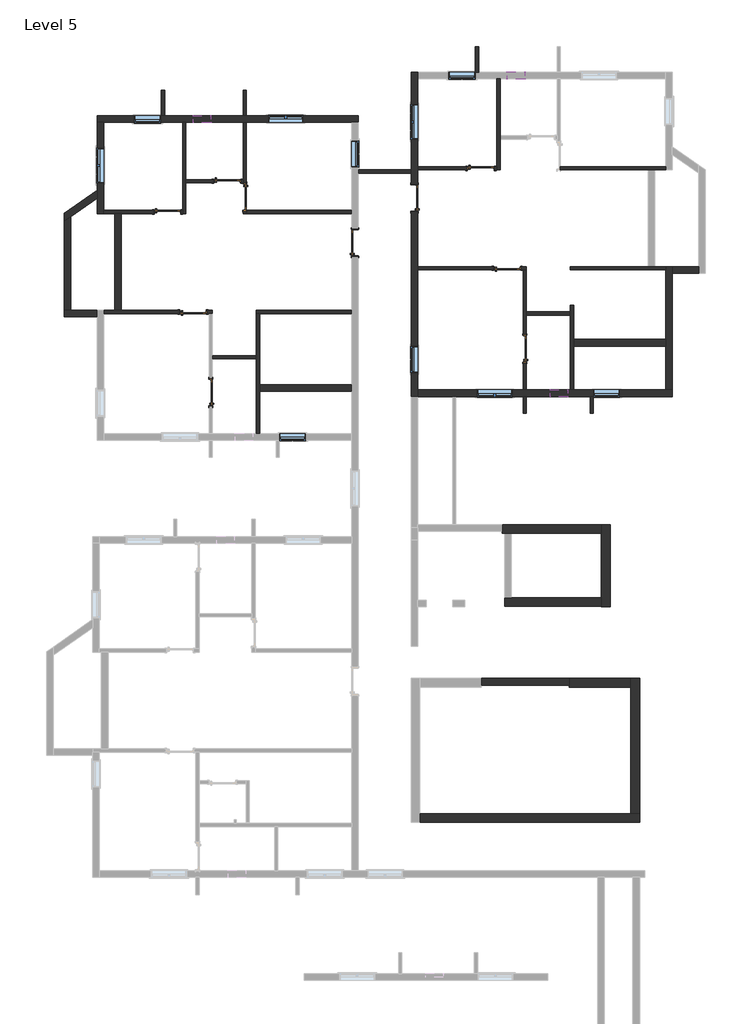
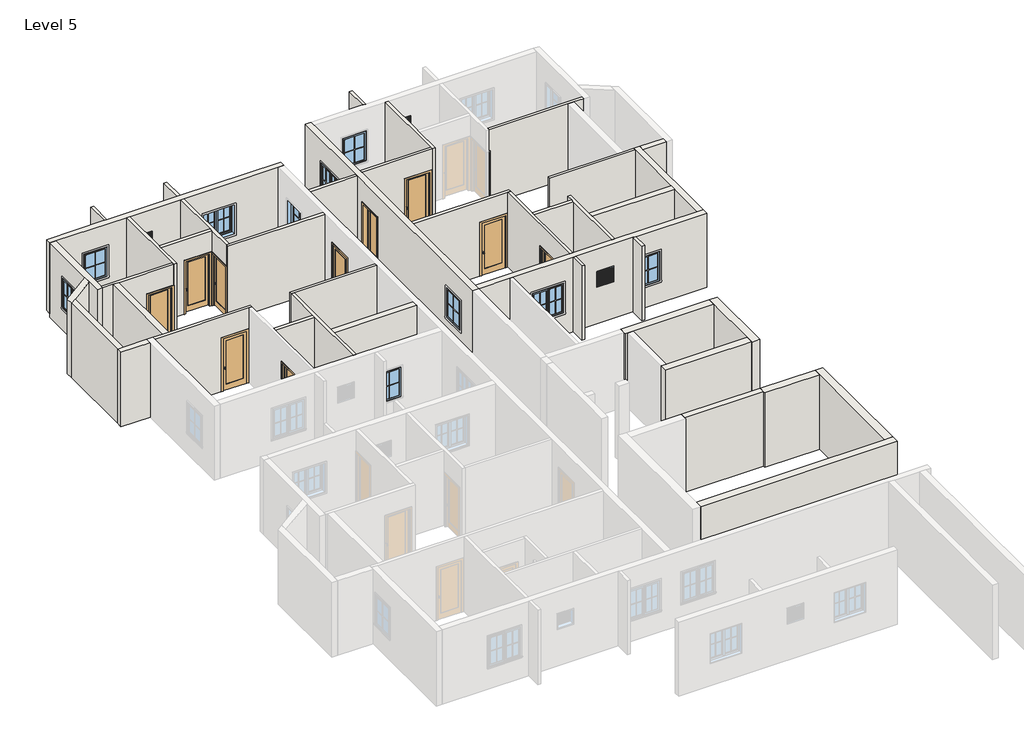
# One storey, part 5 of 7: 42 walls, 13 windows, 10 doors.
"""IFC4 building model written with IfcOpenShell, lengths in millimetres."""

from ifc_helpers import new_model, si_unit, frame, origin, place, context, project, spatial, polyline, outline, extrude, faceted_brep, transform, mapped, element, save
from components import door_3c6ab76a, door_a3feeac7, door_3b97b8e7, door_868ee8a9, window_272f20d6, window_casement_double_4_x_4_af3140d2, window_f2d8fef0

model = new_model("IFC4")

# Units and contexts
model_context = context("Model", 3, world=origin())
ifc_project = project(units=[si_unit("LENGTHUNIT", "METRE", prefix="MILLI")], contexts=[model_context])

# Site, building, storey
site = spatial("IfcSite", under=ifc_project)
building = spatial("IfcBuilding", under=site)
storey = spatial("IfcBuildingStorey", under=building, Name="Level 5", Elevation=6400.8)

# Doors
placement = place(None, origin())
door_shape = door_3c6ab76a(model_context)
element("IfcDoor", 1, ObjectType="Door-Interior-Single-1_Panel-Wood : 2'6\" x 7' door", at=placement, inside=storey, context=model_context, shape_type="MappedRepresentation", body=[
    mapped(door_shape, transform((-10226.9509469, 25492.3711172, 6400.8), x_axis=(1.0, 0.0, 0.0), y_axis=(0.0, 1.0, 0.0), z_axis=(0.0, 0.0, 1.0))),
])
door_2_shape = door_a3feeac7(model_context)
element("IfcDoor", 2, ObjectType="Door-Interior-Single-1_Panel-Wood : 2'6\" x 7' door", at=placement, inside=storey, context=model_context, shape_type="MappedRepresentation", body=[
    mapped(door_2_shape, transform((-10795.2759469, 18161.2961172, 6400.8), x_axis=(0.0, 1.0, 0.0), y_axis=(-1.0, 0.0, 0.0), z_axis=(0.0, 0.0, 1.0))),
])
element("IfcDoor", 3, ObjectType="Door-Interior-Single-1_Panel-Wood : 2'6\" x 7' door", at=placement, inside=storey, context=model_context, shape_type="MappedRepresentation", body=[
    mapped(door_2_shape, transform((101.3240531, 19674.7755084, 6400.8), x_axis=(0.0, 1.0, 0.0), y_axis=(-1.0, 0.0, 0.0), z_axis=(0.0, 0.0, 1.0))),
])
element("IfcDoor", 4, ObjectType="Door-Interior-Single-1_Panel-Wood : 36\" x 84\"", at=placement, inside=storey, context=model_context, shape_type="MappedRepresentation", body=[
    mapped(door_shape, transform((-12297.0509469, 24425.5711172, 6400.8), x_axis=(1.0, 0.0, 0.0), y_axis=(0.0, 1.0, 0.0), z_axis=(0.0, 0.0, 1.0))),
])
element("IfcDoor", 5, ObjectType="Door-Interior-Single-1_Panel-Wood : 36\" x 84\"", at=placement, inside=storey, context=model_context, shape_type="MappedRepresentation", body=[
    mapped(door_shape, transform((-9614.1759469, 24936.7461172, 6400.8), x_axis=(0.0, -1.0, 0.0), y_axis=(1.0, 0.0, 0.0), z_axis=(0.0, 0.0, 1.0))),
])
element("IfcDoor", 6, ObjectType="Door-Interior-Single-1_Panel-Wood : 36\" x 84\"", at=placement, inside=storey, context=model_context, shape_type="MappedRepresentation", body=[
    mapped(door_shape, transform((-1425.8509469, 25939.0505084, 6400.8), x_axis=(1.0, 0.0, 0.0), y_axis=(0.0, 1.0, 0.0), z_axis=(0.0, 0.0, 1.0))),
])
door_3_shape = door_3b97b8e7(model_context)
element("IfcDoor", 7, ObjectType="Door-Interior-Single-1_Panel-Wood : 36\" x 84\"", at=placement, inside=storey, context=model_context, shape_type="MappedRepresentation", body=[
    mapped(door_3_shape, transform((-5791.4759469, 23355.5961172, 6400.8), x_axis=(0.0, 1.0, 0.0), y_axis=(-1.0, 0.0, 0.0), z_axis=(0.0, 0.0, 1.0))),
])
element("IfcDoor", 8, ObjectType="Door-Interior-Single-1_Panel-Wood : 36\" x 84\"", at=placement, inside=storey, context=model_context, shape_type="MappedRepresentation", body=[
    mapped(door_2_shape, transform((-11408.0509469, 20952.1211172, 6400.8), x_axis=(1.0, 0.0, 0.0), y_axis=(0.0, 1.0, 0.0), z_axis=(0.0, 0.0, 1.0))),
])
element("IfcDoor", 9, ObjectType="Door-Interior-Single-1_Panel-Wood : 36\" x 84\"", at=placement, inside=storey, context=model_context, shape_type="MappedRepresentation", body=[
    mapped(door_2_shape, transform((-511.4509469, 22465.6005084, 6400.8), x_axis=(1.0, 0.0, 0.0), y_axis=(0.0, 1.0, 0.0), z_axis=(0.0, 0.0, 1.0))),
])
door_4_shape = door_868ee8a9(model_context)
element("IfcDoor", 10, ObjectType="Door-Interior-Single-1_Panel-Wood : 36\" x 84\"", at=placement, inside=storey, context=model_context, shape_type="MappedRepresentation", body=[
    mapped(door_4_shape, transform((-3727.7259469, 24907.1755084, 6400.8), x_axis=(0.0, 1.0, 0.0), y_axis=(-1.0, 0.0, 0.0), z_axis=(0.0, 0.0, 1.0))),
])

# Walls
element("IfcWall", 11, ObjectType="1' feet", at=placement, inside=storey, context=model_context, shape_type="Brep", body=[
    faceted_brep([(-682.9009469, 13266.6182723, 6400.8), (2758.7990531, 13266.6182723, 6400.8), (2758.7990531, 13266.6182723, 9448.8), (-682.9009469, 13266.6182723, 9448.8), (-682.9009469, 13571.4182723, 6400.8), (-682.9009469, 13571.4182723, 9448.8), (2758.7990531, 13571.4182723, 9448.8), (2758.7990531, 13571.4182723, 6400.8), (-682.9009469, 13342.8182723, 6400.8), (-682.9009469, 13342.8182723, 9448.8)], [[[0, 1, 2, 3]], [[4, 5, 6, 7]], [[1, 0, 8, 4, 7]], [[3, 2, 6, 5, 9]], [[0, 3, 9, 5, 4, 8]], [[2, 1, 7, 6]]]),
])
element("IfcWall", 12, ObjectType="1' feet", at=placement, inside=storey, context=model_context, shape_type="Brep", body=[
    faceted_brep([(3063.5990531, 10726.6182723, 6400.8), (3063.5990531, 13571.4182723, 6400.8), (3063.5990531, 13571.4182723, 9448.8), (3063.5990531, 10726.6182723, 9448.8), (2758.7990531, 10726.6182723, 6400.8), (2758.7990531, 10726.6182723, 9448.8), (2758.7990531, 10739.3182723, 9448.8), (2758.7990531, 11044.1182723, 9448.8), (2758.7990531, 13266.6182723, 9448.8), (2758.7990531, 13571.4182723, 9448.8), (2758.7990531, 13571.4182723, 6400.8), (2758.7990531, 13266.6182723, 6400.8), (2758.7990531, 11044.1182723, 6400.8), (2758.7990531, 10739.3182723, 6400.8)], [[[0, 1, 2, 3]], [[4, 5, 6, 7, 8, 9, 10, 11, 12, 13]], [[1, 0, 4, 13, 12, 11, 10]], [[3, 2, 9, 8, 7, 6, 5]], [[0, 3, 5, 4]], [[2, 1, 10, 9]]]),
])
element("IfcWall", 13, ObjectType="1' feet", at=placement, inside=storey, context=model_context, shape_type="Brep", body=[
    faceted_brep([(2758.7990531, 11044.1182723, 6400.8), (-365.4009469, 11044.1182723, 6400.8), (-594.0009469, 11044.1182723, 6400.8), (-594.0009469, 11044.1182723, 9448.8), (-365.4009469, 11044.1182723, 9448.8), (2758.7990531, 11044.1182723, 9448.8), (2758.7990531, 10739.3182723, 6400.8), (2758.7990531, 10739.3182723, 9448.8), (-594.0009469, 10739.3182723, 9448.8), (-594.0009469, 10739.3182723, 6400.8)], [[[0, 1, 2, 3, 4, 5]], [[6, 7, 8, 9]], [[2, 1, 0, 6, 9]], [[5, 4, 3, 8, 7]], [[0, 5, 7, 6]], [[3, 2, 9, 8]]]),
])
element("IfcWall", 14, ObjectType="1' feet", at=placement, inside=storey, context=model_context, shape_type="Brep", body=[
    faceted_brep([(-3540.4009469, 3245.1461172, 6400.8), (4079.5990531, 3245.1461172, 6400.8), (4079.5990531, 3245.1461172, 9448.8), (-3540.4009469, 3245.1461172, 9448.8), (-3540.4009469, 3549.9461172, 6400.8), (-3540.4009469, 3549.9461172, 9448.8), (3774.7990531, 3549.9461172, 9448.8), (4079.5990531, 3549.9461172, 9448.8), (4079.5990531, 3549.9461172, 6400.8), (3774.7990531, 3549.9461172, 6400.8)], [[[0, 1, 2, 3]], [[4, 5, 6, 7, 8, 9]], [[1, 0, 4, 9, 8]], [[3, 2, 7, 6, 5]], [[2, 1, 8, 7]], [[0, 3, 5, 4]]]),
])
element("IfcWall", 15, ObjectType="1' feet", at=placement, inside=storey, context=model_context, shape_type="Brep", body=[
    faceted_brep([(4079.5990531, 3549.9461172, 6400.8), (4079.5990531, 8236.2461172, 6400.8), (4079.5990531, 8236.2461172, 9448.8), (4079.5990531, 3549.9461172, 9448.8), (3774.7990531, 3549.9461172, 6400.8), (3774.7990531, 3549.9461172, 9448.8), (3774.7990531, 7931.4461172, 9448.8), (3774.7990531, 8236.2461172, 9448.8), (3774.7990531, 8236.2461172, 6400.8), (3774.7990531, 7931.4461172, 6400.8)], [[[0, 1, 2, 3]], [[4, 5, 6, 7, 8, 9]], [[1, 0, 4, 9, 8]], [[3, 2, 7, 6, 5]], [[0, 3, 5, 4]], [[2, 1, 8, 7]]]),
])
element("IfcWall", 16, ObjectType="1' feet", at=placement, inside=storey, context=model_context, shape_type="Brep", body=[
    faceted_brep([(1641.1990531, 7931.4461172, 6400.8), (3774.7990531, 7931.4461172, 6400.8), (3774.7990531, 7931.4461172, 9448.8), (1641.1990531, 7931.4461172, 9448.8), (1641.1990531, 8236.2461172, 6400.8), (1641.1990531, 8236.2461172, 9448.8), (3774.7990531, 8236.2461172, 9448.8), (3774.7990531, 8236.2461172, 6400.8), (1641.1990531, 8007.6461172, 6400.8), (1641.1990531, 8007.6461172, 9448.8)], [[[0, 1, 2, 3]], [[4, 5, 6, 7]], [[1, 0, 8, 4, 7]], [[3, 2, 6, 5, 9]], [[0, 3, 9, 5, 4, 8]], [[2, 1, 7, 6]]]),
])
element("IfcWall", 17, ObjectType="4.5\" wall", at=placement, inside=storey, context=model_context, shape_type="Brep", body=[
    faceted_brep([(-11655.7009469, 24365.2461172, 6400.8), (-11655.7009469, 25432.0461172, 6400.8), (-11655.7009469, 25546.3461172, 6400.8), (-11655.7009469, 27527.5461172, 6400.8), (-11655.7009469, 27527.5461172, 9448.8), (-11655.7009469, 25546.3461172, 9448.8), (-11655.7009469, 25432.0461172, 9448.8), (-11655.7009469, 24365.2461172, 9448.8), (-11770.0009469, 24365.2461172, 6400.8), (-11770.0009469, 24365.2461172, 9448.8), (-11770.0009469, 24479.5461172, 9448.8), (-11770.0009469, 27527.5461172, 9448.8), (-11770.0009469, 27527.5461172, 6400.8), (-11770.0009469, 24479.5461172, 6400.8)], [[[0, 1, 2, 3, 4, 5, 6, 7]], [[8, 9, 10, 11, 12, 13]], [[3, 2, 1, 0, 8, 13, 12]], [[7, 6, 5, 4, 11, 10, 9]], [[4, 3, 12, 11]], [[0, 7, 9, 8]]]),
])
element("IfcWall", 18, ObjectType="4.5\" wall", at=placement, inside=storey, context=model_context, shape_type="SweptSolid", body=[
    extrude(outline(polyline([(9448.8, -9674.5009469), (9448.8, -11655.7009469), (6400.8, -11655.7009469), (6400.8, -10709.5509469), (8559.8, -10709.5509469), (8559.8, -9744.3509469), (6400.8, -9744.3509469), (6400.8, -9674.5009469), (9448.8, -9674.5009469)])), frame((0.0, 25432.0461172, 0.0), z_axis=(0.0, 1.0, 0.0), x_axis=(0.0, 0.0, 1.0)), (0.0, 0.0, 1.0), 114.3),
])
element("IfcWall", 19, ObjectType="4.5\" wall", at=placement, inside=storey, context=model_context, shape_type="Brep", body=[
    faceted_brep([(-11770.0009469, 24365.2461172, 9448.8), (-13903.6009469, 24365.2461172, 9448.8), (-14132.2009469, 24365.2461172, 9448.8), (-14513.2009469, 24365.2461172, 9448.8), (-14513.2009469, 24365.2461172, 6400.8), (-14132.2009469, 24365.2461172, 6400.8), (-13903.6009469, 24365.2461172, 6400.8), (-12779.6509469, 24365.2461172, 6400.8), (-12779.6509469, 24365.2461172, 8559.8), (-11814.4509469, 24365.2461172, 8559.8), (-11814.4509469, 24365.2461172, 6400.8), (-11770.0009469, 24365.2461172, 6400.8), (-14513.2009469, 24479.5461172, 9448.8), (-11770.0009469, 24479.5461172, 9448.8), (-11770.0009469, 24479.5461172, 6400.8), (-11814.4509469, 24479.5461172, 6400.8), (-11814.4509469, 24479.5461172, 8559.8), (-12779.6509469, 24479.5461172, 8559.8), (-12779.6509469, 24479.5461172, 6400.8), (-14513.2009469, 24479.5461172, 6400.8)], [[[0, 1, 2, 3, 4, 5, 6, 7, 8, 9, 10, 11]], [[12, 13, 14, 15, 16, 17, 18, 19]], [[4, 19, 18, 7, 6, 5]], [[14, 11, 10, 15]], [[3, 2, 1, 0, 13, 12]], [[4, 3, 12, 19]], [[0, 11, 14, 13]], [[9, 16, 15, 10]], [[16, 9, 8, 17]], [[17, 8, 7, 18]]]),
])
element("IfcWall", 20, ObjectType="4.5\" wall", at=placement, inside=storey, context=model_context, shape_type="Brep", body=[
    faceted_brep([(-9674.5009469, 24479.5461172, 9448.8), (-9560.2009469, 24479.5461172, 9448.8), (-5902.6009469, 24479.5461172, 9448.8), (-5902.6009469, 24479.5461172, 6400.8), (-9560.2009469, 24479.5461172, 6400.8), (-9560.2009469, 24479.5461172, 8559.8), (-9674.5009469, 24479.5461172, 8559.8), (-9674.5009469, 24365.2461172, 6400.8), (-5902.6009469, 24365.2461172, 6400.8), (-5902.6009469, 24365.2461172, 9448.8), (-9674.5009469, 24365.2461172, 9448.8), (-9674.5009469, 24454.1461172, 6400.8), (-9560.2009469, 24454.1461172, 6400.8), (-9674.5009469, 24454.1461172, 8559.8), (-9560.2009469, 24454.1461172, 8559.8)], [[[0, 1, 2, 3, 4, 5, 6]], [[7, 8, 9, 10]], [[8, 7, 11, 12, 4, 3]], [[2, 1, 0, 10, 9]], [[7, 10, 0, 6, 13, 11]], [[3, 2, 9, 8]], [[12, 14, 5, 4]], [[14, 12, 11, 13]], [[14, 13, 6, 5]]]),
])
element("IfcWall", 21, ObjectType="4.5\" wall", at=placement, inside=storey, context=model_context, shape_type="Brep", body=[
    faceted_brep([(-5902.6009469, 21012.4461172, 6400.8), (-9217.3009469, 21012.4461172, 6400.8), (-9217.3009469, 21012.4461172, 9448.8), (-5902.6009469, 21012.4461172, 9448.8), (-5902.6009469, 20898.1461172, 6400.8), (-5902.6009469, 20898.1461172, 9448.8), (-9103.0009469, 20898.1461172, 9448.8), (-9217.3009469, 20898.1461172, 9448.8), (-9217.3009469, 20898.1461172, 6400.8), (-9103.0009469, 20898.1461172, 6400.8)], [[[0, 1, 2, 3]], [[4, 5, 6, 7, 8, 9]], [[1, 0, 4, 9, 8]], [[3, 2, 7, 6, 5]], [[0, 3, 5, 4]], [[2, 1, 8, 7]]]),
])
element("IfcWall", 22, ObjectType="4.5\" wall", at=placement, inside=storey, context=model_context, shape_type="Brep", body=[
    faceted_brep([(-14513.2009469, 21012.4461172, 9448.8), (-14132.2009469, 21012.4461172, 9448.8), (-13903.6009469, 21012.4461172, 9448.8), (-10741.3009469, 21012.4461172, 9448.8), (-10741.3009469, 21012.4461172, 6400.8), (-10925.4509469, 21012.4461172, 6400.8), (-10925.4509469, 21012.4461172, 8559.8), (-11890.6509469, 21012.4461172, 8559.8), (-11890.6509469, 21012.4461172, 6400.8), (-13903.6009469, 21012.4461172, 6400.8), (-14132.2009469, 21012.4461172, 6400.8), (-14513.2009469, 21012.4461172, 6400.8), (-10741.3009469, 20898.1461172, 9448.8), (-10855.6009469, 20898.1461172, 9448.8), (-14513.2009469, 20898.1461172, 9448.8), (-14513.2009469, 20898.1461172, 6400.8), (-11890.6509469, 20898.1461172, 6400.8), (-11890.6509469, 20898.1461172, 8559.8), (-10925.4509469, 20898.1461172, 8559.8), (-10925.4509469, 20898.1461172, 6400.8), (-10855.6009469, 20898.1461172, 6400.8), (-10741.3009469, 20898.1461172, 6400.8)], [[[0, 1, 2, 3, 4, 5, 6, 7, 8, 9, 10, 11]], [[12, 13, 14, 15, 16, 17, 18, 19, 20, 21]], [[15, 11, 10, 9, 8, 16]], [[4, 21, 20, 19, 5]], [[3, 2, 1, 0, 14, 13, 12]], [[0, 11, 15, 14]], [[4, 3, 12, 21]], [[18, 6, 5, 19]], [[6, 18, 17, 7]], [[7, 17, 16, 8]]]),
])
element("IfcWall", 23, ObjectType="4.5\" wall", at=placement, inside=storey, context=model_context, shape_type="Brep", body=[
    faceted_brep([(-9560.2009469, 27527.5461172, 9448.8), (-9560.2009469, 24479.5461172, 9448.8), (-9560.2009469, 24479.5461172, 8559.8), (-9560.2009469, 25419.3461172, 8559.8), (-9560.2009469, 25419.3461172, 6400.8), (-9560.2009469, 27527.5461172, 6400.8), (-9674.5009469, 24479.5461172, 9448.8), (-9674.5009469, 25432.0461172, 9448.8), (-9674.5009469, 25546.3461172, 9448.8), (-9674.5009469, 27527.5461172, 9448.8), (-9674.5009469, 27527.5461172, 6400.8), (-9674.5009469, 25546.3461172, 6400.8), (-9674.5009469, 25432.0461172, 6400.8), (-9674.5009469, 25419.3461172, 6400.8), (-9674.5009469, 25419.3461172, 8559.8), (-9674.5009469, 24479.5461172, 8559.8)], [[[0, 1, 2, 3, 4, 5]], [[6, 7, 8, 9, 10, 11, 12, 13, 14, 15]], [[10, 5, 4, 13, 12, 11]], [[1, 0, 9, 8, 7, 6]], [[0, 5, 10, 9]], [[1, 6, 15, 2]], [[14, 3, 2, 15]], [[3, 14, 13, 4]]]),
])
element("IfcWall", 24, ObjectType="4.5\" wall", at=placement, inside=storey, context=model_context, shape_type="SweptSolid", body=[
    extrude(outline(polyline([(-9217.3009469, 19323.3461172), (-10741.3009469, 19323.3461172), (-10741.3009469, 19437.6461172), (-9217.3009469, 19437.6461172), (-9217.3009469, 19323.3461172)])), frame((0.0, 0.0, 6400.8), z_axis=(0.0, 0.0, 1.0), x_axis=(1.0, 0.0, 0.0)), (0.0, 0.0, 1.0), 3048.0),
])
element("IfcWall", 25, ObjectType="4.5\" wall", at=placement, inside=storey, context=model_context, shape_type="Brep", body=[
    faceted_brep([(-9217.3009469, 20898.1461172, 6400.8), (-9217.3009469, 19437.6461172, 6400.8), (-9217.3009469, 19323.3461172, 6400.8), (-9217.3009469, 16732.5461172, 6400.8), (-9217.3009469, 16732.5461172, 9448.8), (-9217.3009469, 19323.3461172, 9448.8), (-9217.3009469, 19437.6461172, 9448.8), (-9217.3009469, 20898.1461172, 9448.8), (-9103.0009469, 20898.1461172, 6400.8), (-9103.0009469, 20898.1461172, 9448.8), (-9103.0009469, 18434.3461172, 9448.8), (-9103.0009469, 18205.7461172, 9448.8), (-9103.0009469, 16732.5461172, 9448.8), (-9103.0009469, 16732.5461172, 6400.8), (-9103.0009469, 18205.7461172, 6400.8), (-9103.0009469, 18434.3461172, 6400.8)], [[[0, 1, 2, 3, 4, 5, 6, 7]], [[8, 9, 10, 11, 12, 13, 14, 15]], [[3, 2, 1, 0, 8, 15, 14, 13]], [[7, 6, 5, 4, 12, 11, 10, 9]], [[0, 7, 9, 8]], [[4, 3, 13, 12]]]),
])
element("IfcWall", 26, ObjectType="4.5\" wall", at=placement, inside=storey, context=model_context, shape_type="SweptSolid", body=[
    extrude(outline(polyline([(-5674.0009469, 25878.7255084), (-3845.2009469, 25878.7255084), (-3845.2009469, 25764.4255084), (-5674.0009469, 25764.4255084), (-5674.0009469, 25878.7255084)])), frame((0.0, 0.0, 6400.8), z_axis=(0.0, 0.0, 1.0), x_axis=(1.0, 0.0, 0.0)), (0.0, 0.0, 1.0), 3048.0),
])
element("IfcWall", 27, ObjectType="4.5\" wall", at=placement, inside=storey, context=model_context, shape_type="Brep", body=[
    faceted_brep([(-759.1009469, 25878.7255084, 6400.8), (-759.1009469, 26945.5255084, 6400.8), (-759.1009469, 27059.8255084, 6400.8), (-759.1009469, 29041.0255084, 6400.8), (-759.1009469, 29041.0255084, 9448.8), (-759.1009469, 27059.8255084, 9448.8), (-759.1009469, 26945.5255084, 9448.8), (-759.1009469, 25878.7255084, 9448.8), (-873.4009469, 25878.7255084, 6400.8), (-873.4009469, 25878.7255084, 9448.8), (-873.4009469, 25993.0255084, 9448.8), (-873.4009469, 29041.0255084, 9448.8), (-873.4009469, 29041.0255084, 6400.8), (-873.4009469, 25993.0255084, 6400.8)], [[[0, 1, 2, 3, 4, 5, 6, 7]], [[8, 9, 10, 11, 12, 13]], [[3, 2, 1, 0, 8, 13, 12]], [[7, 6, 5, 4, 11, 10, 9]], [[4, 3, 12, 11]], [[0, 7, 9, 8]]]),
])
element("IfcWall", 28, ObjectType="4.5\" wall", at=placement, inside=storey, context=model_context, shape_type="SweptSolid", body=[
    extrude(outline(polyline([(9448.8, -873.4009469), (9448.8, -3616.6009469), (6400.8, -3616.6009469), (6400.8, -1908.4509469), (8559.8, -1908.4509469), (8559.8, -943.2509469), (6400.8, -943.2509469), (6400.8, -873.4009469), (9448.8, -873.4009469)])), frame((0.0, 25878.7255084, 0.0), z_axis=(0.0, 1.0, 0.0), x_axis=(0.0, 0.0, 1.0)), (0.0, 0.0, 1.0), 114.3),
])
element("IfcWall", 29, ObjectType="4.5\" wall", at=placement, inside=storey, context=model_context, shape_type="Brep", body=[
    faceted_brep([(4993.9990531, 25993.0255084, 6400.8), (1336.3990531, 25993.0255084, 6400.8), (1336.3990531, 25993.0255084, 9448.8), (4993.9990531, 25993.0255084, 9448.8), (4993.9990531, 25878.7255084, 6400.8), (4993.9990531, 25878.7255084, 9448.8), (4612.9990531, 25878.7255084, 9448.8), (4384.3990531, 25878.7255084, 9448.8), (1336.3990531, 25878.7255084, 9448.8), (1336.3990531, 25878.7255084, 6400.8), (4384.3990531, 25878.7255084, 6400.8), (4612.9990531, 25878.7255084, 6400.8)], [[[0, 1, 2, 3]], [[4, 5, 6, 7, 8, 9, 10, 11]], [[1, 0, 4, 11, 10, 9]], [[3, 2, 8, 7, 6, 5]], [[2, 1, 9, 8]], [[0, 3, 5, 4]]]),
])
element("IfcWall", 30, ObjectType="4.5\" wall", at=placement, inside=storey, context=model_context, shape_type="Brep", body=[
    faceted_brep([(4993.9990531, 22525.9255084, 6400.8), (4612.9990531, 22525.9255084, 6400.8), (4384.3990531, 22525.9255084, 6400.8), (1679.2990531, 22525.9255084, 6400.8), (1679.2990531, 22525.9255084, 9448.8), (4384.3990531, 22525.9255084, 9448.8), (4612.9990531, 22525.9255084, 9448.8), (4993.9990531, 22525.9255084, 9448.8), (4993.9990531, 22411.6255084, 6400.8), (4993.9990531, 22411.6255084, 9448.8), (1679.2990531, 22411.6255084, 9448.8), (1679.2990531, 22411.6255084, 6400.8)], [[[0, 1, 2, 3, 4, 5, 6, 7]], [[8, 9, 10, 11]], [[3, 2, 1, 0, 8, 11]], [[4, 3, 11, 10]], [[7, 6, 5, 4, 10, 9]], [[0, 7, 9, 8]]]),
])
element("IfcWall", 31, ObjectType="4.5\" wall", at=placement, inside=storey, context=model_context, shape_type="Brep", body=[
    faceted_brep([(155.2990531, 22411.6255084, 9448.8), (40.9990531, 22411.6255084, 9448.8), (-3616.6009469, 22411.6255084, 9448.8), (-3616.6009469, 22411.6255084, 6400.8), (-994.0509469, 22411.6255084, 6400.8), (-994.0509469, 22411.6255084, 8559.8), (-28.8509469, 22411.6255084, 8559.8), (-28.8509469, 22411.6255084, 6400.8), (40.9990531, 22411.6255084, 6400.8), (155.2990531, 22411.6255084, 6400.8), (-3616.6009469, 22525.9255084, 9448.8), (155.2990531, 22525.9255084, 9448.8), (155.2990531, 22525.9255084, 6400.8), (-28.8509469, 22525.9255084, 6400.8), (-28.8509469, 22525.9255084, 8559.8), (-994.0509469, 22525.9255084, 8559.8), (-994.0509469, 22525.9255084, 6400.8), (-3616.6009469, 22525.9255084, 6400.8)], [[[0, 1, 2, 3, 4, 5, 6, 7, 8, 9]], [[10, 11, 12, 13, 14, 15, 16, 17]], [[3, 17, 16, 4]], [[12, 9, 8, 7, 13]], [[2, 1, 0, 11, 10]], [[3, 2, 10, 17]], [[0, 9, 12, 11]], [[6, 14, 13, 7]], [[14, 6, 5, 15]], [[15, 5, 4, 16]]]),
])
element("IfcWall", 32, ObjectType="4.5\" wall", at=placement, inside=storey, context=model_context, shape_type="Brep", body=[
    faceted_brep([(155.2990531, 22411.6255084, 9448.8), (155.2990531, 20951.1255084, 9448.8), (155.2990531, 20836.8255084, 9448.8), (155.2990531, 18246.0255084, 9448.8), (155.2990531, 18246.0255084, 6400.8), (155.2990531, 19192.1755084, 6400.8), (155.2990531, 19192.1755084, 8559.8), (155.2990531, 20157.3755084, 8559.8), (155.2990531, 20157.3755084, 6400.8), (155.2990531, 20836.8255084, 6400.8), (155.2990531, 20951.1255084, 6400.8), (155.2990531, 22411.6255084, 6400.8), (40.9990531, 18246.0255084, 9448.8), (40.9990531, 22411.6255084, 9448.8), (40.9990531, 22411.6255084, 6400.8), (40.9990531, 20157.3755084, 6400.8), (40.9990531, 20157.3755084, 8559.8), (40.9990531, 19192.1755084, 8559.8), (40.9990531, 19192.1755084, 6400.8), (40.9990531, 18246.0255084, 6400.8)], [[[0, 1, 2, 3, 4, 5, 6, 7, 8, 9, 10, 11]], [[12, 13, 14, 15, 16, 17, 18, 19]], [[14, 11, 10, 9, 8, 15]], [[4, 19, 18, 5]], [[3, 2, 1, 0, 13, 12]], [[0, 11, 14, 13]], [[4, 3, 12, 19]], [[7, 16, 15, 8]], [[16, 7, 6, 17]], [[17, 6, 5, 18]]]),
])
element("IfcWall", 33, ObjectType="4.5\" wall", at=placement, inside=storey, context=model_context, shape_type="Brep", body=[
    faceted_brep([(1679.2990531, 21192.4255084, 6400.8), (1679.2990531, 20951.1255084, 6400.8), (1679.2990531, 20836.8255084, 6400.8), (1679.2990531, 18246.0255084, 6400.8), (1679.2990531, 18246.0255084, 9448.8), (1679.2990531, 20836.8255084, 9448.8), (1679.2990531, 20951.1255084, 9448.8), (1679.2990531, 21192.4255084, 9448.8), (1793.5990531, 21192.4255084, 6400.8), (1793.5990531, 21192.4255084, 9448.8), (1793.5990531, 19998.6255084, 9448.8), (1793.5990531, 19770.0255084, 9448.8), (1793.5990531, 18246.0255084, 9448.8), (1793.5990531, 18246.0255084, 6400.8), (1793.5990531, 19770.0255084, 6400.8), (1793.5990531, 19998.6255084, 6400.8)], [[[0, 1, 2, 3, 4, 5, 6, 7]], [[8, 9, 10, 11, 12, 13, 14, 15]], [[3, 2, 1, 0, 8, 15, 14, 13]], [[7, 6, 5, 4, 12, 11, 10, 9]], [[0, 7, 9, 8]], [[4, 3, 13, 12]]]),
])
element("IfcWall", 34, ObjectType="4.5\" wall", at=placement, inside=storey, context=model_context, shape_type="SweptSolid", body=[
    extrude(outline(polyline([(155.2990531, 20951.1255084), (1679.2990531, 20951.1255084), (1679.2990531, 20836.8255084), (155.2990531, 20836.8255084), (155.2990531, 20951.1255084)])), frame((0.0, 0.0, 6400.8), z_axis=(0.0, 0.0, 1.0), x_axis=(1.0, 0.0, 0.0)), (0.0, 0.0, 1.0), 3048.0),
])
element("IfcWall", 35, ObjectType="4.5\" wall", at=placement, inside=storey, context=model_context, shape_type="Brep", body=[
    faceted_brep([(-1617.8862554, 30161.6889788, 6400.8), (-1617.8862554, 29269.6255084, 6400.8), (-1617.8862554, 29269.6255084, 7315.2), (-1617.8862554, 29269.6255084, 8534.4), (-1617.8862554, 29269.6255084, 9448.8), (-1617.8862554, 30161.6889788, 9448.8), (-1503.5862554, 30161.6889788, 6400.8), (-1503.5862554, 30161.6889788, 9448.8), (-1503.5862554, 29269.6255084, 9448.8), (-1503.5862554, 29269.6255084, 6400.8)], [[[0, 1, 2, 3, 4, 5]], [[6, 7, 8, 9]], [[1, 0, 6, 9]], [[5, 4, 8, 7]], [[0, 5, 7, 6]], [[4, 3, 2, 1, 9, 8]]]),
])
element("IfcWall", 36, ObjectType="4.5\" wall", at=placement, inside=storey, context=model_context, shape_type="SweptSolid", body=[
    extrude(outline(polyline([(40.9990531, 17431.8689406), (40.9990531, 18017.4255084), (155.2990531, 18017.4255084), (155.2990531, 17431.8689406), (40.9990531, 17431.8689406)])), frame((0.0, 0.0, 6400.8), z_axis=(0.0, 0.0, 1.0), x_axis=(1.0, 0.0, 0.0)), (0.0, 0.0, 1.0), 3048.0),
])
element("IfcWall", 37, ObjectType="4.5\" wall", at=placement, inside=storey, context=model_context, shape_type="Brep", body=[
    faceted_brep([(2365.0990531, 18017.4255084, 6400.8), (2365.0990531, 17431.8689406, 6400.8), (2365.0990531, 17431.8689406, 9448.8), (2365.0990531, 18017.4255084, 9448.8), (2479.3990531, 18017.4255084, 6400.8), (2479.3990531, 18017.4255084, 7315.2), (2479.3990531, 18017.4255084, 8534.4), (2479.3990531, 18017.4255084, 9448.8), (2479.3990531, 17431.8689406, 9448.8), (2479.3990531, 17431.8689406, 6400.8)], [[[0, 1, 2, 3]], [[4, 5, 6, 7, 8, 9]], [[1, 0, 4, 9]], [[2, 1, 9, 8]], [[3, 2, 8, 7]], [[0, 3, 7, 6, 5, 4]]]),
])
element("IfcWall", 38, ObjectType="4.5\" wall", at=placement, inside=storey, context=model_context, shape_type="SweptSolid", body=[
    extrude(outline(polyline([(-12514.4862554, 27756.1461172), (-12514.4862554, 28648.2095876), (-12400.1862554, 28648.2095876), (-12400.1862554, 27756.1461172), (-12514.4862554, 27756.1461172)])), frame((0.0, 0.0, 6400.8), z_axis=(0.0, 0.0, 1.0), x_axis=(1.0, 0.0, 0.0)), (0.0, 0.0, 1.0), 3048.0),
])
element("IfcWall", 39, ObjectType="4.5\" wall", at=placement, inside=storey, context=model_context, shape_type="SweptSolid", body=[
    extrude(outline(polyline([(-9560.2009469, 28648.2095876), (-9560.2009469, 27756.1461172), (-9674.5009469, 27756.1461172), (-9674.5009469, 28648.2095876), (-9560.2009469, 28648.2095876)])), frame((0.0, 0.0, 6400.8), z_axis=(0.0, 0.0, 1.0), x_axis=(1.0, 0.0, 0.0)), (0.0, 0.0, 1.0), 3048.0),
])
element("IfcWall", 40, ObjectType="9\"", at=placement, inside=storey, context=model_context, shape_type="Brep", body=[
    faceted_brep([(-5674.0009469, 27756.1461172, 6553.2), (-14741.8009469, 27756.1461172, 6553.2), (-14741.8009469, 27756.1461172, 9448.8), (-12514.4862554, 27756.1461172, 9448.8), (-12400.1862554, 27756.1461172, 9448.8), (-9674.5009469, 27756.1461172, 9448.8), (-9560.2009469, 27756.1461172, 9448.8), (-5674.0009469, 27756.1461172, 9448.8), (-10798.4509469, 27756.1461172, 8534.4), (-11408.0509469, 27756.1461172, 8534.4), (-11408.0509469, 27756.1461172, 7924.8), (-10798.4509469, 27756.1461172, 7924.8), (-13447.9362554, 27756.1461172, 8534.4), (-13447.9362554, 27756.1461172, 7315.2), (-12533.5362554, 27756.1461172, 7315.2), (-12533.5362554, 27756.1461172, 8534.4), (-7585.3509469, 27756.1461172, 8534.4), (-8804.5509469, 27756.1461172, 8534.4), (-8804.5509469, 27756.1461172, 7315.2), (-7585.3509469, 27756.1461172, 7315.2), (-5674.0009469, 27527.5461172, 6553.2), (-5674.0009469, 27527.5461172, 9448.8), (-5902.6009469, 27527.5461172, 9448.8), (-9560.2009469, 27527.5461172, 9448.8), (-9674.5009469, 27527.5461172, 9448.8), (-11655.7009469, 27527.5461172, 9448.8), (-11770.0009469, 27527.5461172, 9448.8), (-14513.2009469, 27527.5461172, 9448.8), (-14741.8009469, 27527.5461172, 9448.8), (-14741.8009469, 27527.5461172, 6553.2), (-10798.4509469, 27527.5461172, 8534.4), (-10798.4509469, 27527.5461172, 7924.8), (-11408.0509469, 27527.5461172, 7924.8), (-11408.0509469, 27527.5461172, 8534.4), (-13447.9362554, 27527.5461172, 8534.4), (-12533.5362554, 27527.5461172, 8534.4), (-12533.5362554, 27527.5461172, 7315.2), (-13447.9362554, 27527.5461172, 7315.2), (-7585.3509469, 27527.5461172, 8534.4), (-7585.3509469, 27527.5461172, 7315.2), (-8804.5509469, 27527.5461172, 7315.2), (-8804.5509469, 27527.5461172, 8534.4)], [[[0, 1, 2, 3, 4, 5, 6, 7], [8, 9, 10, 11], [12, 13, 14, 15], [16, 17, 18, 19]], [[20, 21, 22, 23, 24, 25, 26, 27, 28, 29], [30, 31, 32, 33], [34, 35, 36, 37], [38, 39, 40, 41]], [[1, 0, 20, 29]], [[7, 6, 5, 4, 3, 2, 28, 27, 26, 25, 24, 23, 22, 21]], [[2, 1, 29, 28]], [[0, 7, 21, 20]], [[31, 30, 8, 11]], [[32, 31, 11, 10]], [[33, 32, 10, 9]], [[30, 33, 9, 8]], [[13, 12, 34, 37]], [[14, 13, 37, 36]], [[15, 14, 36, 35]], [[12, 15, 35, 34]], [[39, 38, 16, 19]], [[40, 39, 19, 18]], [[41, 40, 18, 17]], [[38, 41, 17, 16]]]),
])
element("IfcWall", 41, ObjectType="9\"", at=placement, inside=storey, context=model_context, shape_type="Brep", body=[
    faceted_brep([(-14741.8009469, 27527.5461172, 6400.8), (-14741.8009469, 25177.6879786, 6400.8), (-14741.8009469, 24898.6461172, 6400.8), (-14741.8009469, 24365.2461172, 6400.8), (-14741.8009469, 24365.2461172, 9448.8), (-14741.8009469, 24898.6461172, 9448.8), (-14741.8009469, 25177.6879786, 9448.8), (-14741.8009469, 27527.5461172, 9448.8), (-14741.8009469, 27527.5461172, 6553.2), (-14741.8009469, 26641.7211172, 8534.4), (-14741.8009469, 25422.5211172, 8534.4), (-14741.8009469, 25422.5211172, 7315.2), (-14741.8009469, 26641.7211172, 7315.2), (-14513.2009469, 27527.5461172, 6400.8), (-14513.2009469, 27527.5461172, 9448.8), (-14513.2009469, 24479.5461172, 9448.8), (-14513.2009469, 24365.2461172, 9448.8), (-14513.2009469, 24365.2461172, 6400.8), (-14513.2009469, 24479.5461172, 6400.8), (-14513.2009469, 26641.7211172, 8534.4), (-14513.2009469, 26641.7211172, 7315.2), (-14513.2009469, 25422.5211172, 7315.2), (-14513.2009469, 25422.5211172, 8534.4)], [[[0, 1, 2, 3, 4, 5, 6, 7, 8], [9, 10, 11, 12]], [[13, 14, 15, 16, 17, 18], [19, 20, 21, 22]], [[3, 2, 1, 0, 13, 18, 17]], [[7, 6, 5, 4, 16, 15, 14]], [[0, 8, 7, 14, 13]], [[4, 3, 17, 16]], [[20, 19, 9, 12]], [[21, 20, 12, 11]], [[22, 21, 11, 10]], [[19, 22, 10, 9]]]),
])
element("IfcWall", 42, ObjectType="9\"", at=placement, inside=storey, context=model_context, shape_type="SweptSolid", body=[
    extrude(outline(polyline([(-13903.6009469, 24365.2461172), (-13903.6009469, 21012.4461172), (-14132.2009469, 21012.4461172), (-14132.2009469, 24365.2461172), (-13903.6009469, 24365.2461172)])), frame((0.0, 0.0, 6400.8), z_axis=(0.0, 0.0, 1.0), x_axis=(1.0, 0.0, 0.0)), (0.0, 0.0, 1.0), 3048.0),
])
element("IfcWall", 43, ObjectType="9\"", at=placement, inside=storey, context=model_context, shape_type="SweptSolid", body=[
    extrude(outline(polyline([(-5902.6009469, 18205.7461172), (-9103.0009469, 18205.7461172), (-9103.0009469, 18434.3461172), (-5902.6009469, 18434.3461172), (-5902.6009469, 18205.7461172)])), frame((0.0, 0.0, 6400.8), z_axis=(0.0, 0.0, 1.0), x_axis=(1.0, 0.0, 0.0)), (0.0, 0.0, 1.0), 3048.0),
])
element("IfcWall", 44, ObjectType="9\"", at=placement, inside=storey, context=model_context, shape_type="Brep", body=[
    faceted_brep([(-3616.6009469, 29269.6255084, 9448.8), (-3616.6009469, 29041.0255084, 9448.8), (-3616.6009469, 25993.0255084, 9448.8), (-3616.6009469, 25878.7255084, 9448.8), (-3616.6009469, 22525.9255084, 9448.8), (-3616.6009469, 22411.6255084, 9448.8), (-3616.6009469, 18246.0255084, 9448.8), (-3616.6009469, 18017.4255084, 9448.8), (-3616.6009469, 18017.4255084, 6400.8), (-3616.6009469, 18246.0255084, 6400.8), (-3616.6009469, 22411.6255084, 6400.8), (-3616.6009469, 22525.9255084, 6400.8), (-3616.6009469, 24424.5755084, 6400.8), (-3616.6009469, 24424.5755084, 8559.8), (-3616.6009469, 25389.7755084, 8559.8), (-3616.6009469, 25389.7755084, 6400.8), (-3616.6009469, 25878.7255084, 6400.8), (-3616.6009469, 25993.0255084, 6400.8), (-3616.6009469, 29041.0255084, 6400.8), (-3616.6009469, 29269.6255084, 6400.8), (-3616.6009469, 19757.3255084, 8534.4), (-3616.6009469, 19757.3255084, 7315.2), (-3616.6009469, 18842.9255084, 7315.2), (-3616.6009469, 18842.9255084, 8534.4), (-3616.6009469, 28155.2005084, 8534.4), (-3616.6009469, 28155.2005084, 7315.2), (-3616.6009469, 26936.0005084, 7315.2), (-3616.6009469, 26936.0005084, 8534.4), (-3845.2009469, 18017.4255084, 9448.8), (-3845.2009469, 25764.4255084, 9448.8), (-3845.2009469, 25878.7255084, 9448.8), (-3845.2009469, 29269.6255084, 9448.8), (-3845.2009469, 29269.6255084, 6400.8), (-3845.2009469, 25878.7255084, 6400.8), (-3845.2009469, 25764.4255084, 6400.8), (-3845.2009469, 25389.7755084, 6400.8), (-3845.2009469, 25389.7755084, 8559.8), (-3845.2009469, 24424.5755084, 8559.8), (-3845.2009469, 24424.5755084, 6400.8), (-3845.2009469, 18017.4255084, 6400.8), (-3845.2009469, 19757.3255084, 8534.4), (-3845.2009469, 18842.9255084, 8534.4), (-3845.2009469, 18842.9255084, 7315.2), (-3845.2009469, 19757.3255084, 7315.2), (-3845.2009469, 28155.2005084, 8534.4), (-3845.2009469, 26936.0005084, 8534.4), (-3845.2009469, 26936.0005084, 7315.2), (-3845.2009469, 28155.2005084, 7315.2)], [[[0, 1, 2, 3, 4, 5, 6, 7, 8, 9, 10, 11, 12, 13, 14, 15, 16, 17, 18, 19], [20, 21, 22, 23], [24, 25, 26, 27]], [[28, 29, 30, 31, 32, 33, 34, 35, 36, 37, 38, 39], [40, 41, 42, 43], [44, 45, 46, 47]], [[32, 19, 18, 17, 16, 15, 35, 34, 33]], [[8, 39, 38, 12, 11, 10, 9]], [[7, 6, 5, 4, 3, 2, 1, 0, 31, 30, 29, 28]], [[0, 19, 32, 31]], [[8, 7, 28, 39]], [[14, 36, 35, 15]], [[36, 14, 13, 37]], [[37, 13, 12, 38]], [[21, 20, 40, 43]], [[22, 21, 43, 42]], [[23, 22, 42, 41]], [[20, 23, 41, 40]], [[25, 24, 44, 47]], [[26, 25, 47, 46]], [[27, 26, 46, 45]], [[24, 27, 45, 44]]]),
])
element("IfcWall", 45, ObjectType="9\"", at=placement, inside=storey, context=model_context, shape_type="Brep", body=[
    faceted_brep([(-3616.6009469, 18017.4255084, 6400.8), (-2402.381873, 18017.4255084, 6400.8), (-2288.081873, 18017.4255084, 6400.8), (40.9990531, 18017.4255084, 6400.8), (155.2990531, 18017.4255084, 6400.8), (2365.0990531, 18017.4255084, 6400.8), (2479.3990531, 18017.4255084, 6400.8), (5222.5990531, 18017.4255084, 6400.8), (5222.5990531, 18017.4255084, 9448.8), (2479.3990531, 18017.4255084, 9448.8), (2365.0990531, 18017.4255084, 9448.8), (155.2990531, 18017.4255084, 9448.8), (40.9990531, 18017.4255084, 9448.8), (-2288.081873, 18017.4255084, 9448.8), (-2402.381873, 18017.4255084, 9448.8), (-3616.6009469, 18017.4255084, 9448.8), (1590.3990531, 18017.4255084, 8534.4), (1590.3990531, 18017.4255084, 7924.8), (980.7990531, 18017.4255084, 7924.8), (980.7990531, 18017.4255084, 8534.4), (2479.3990531, 18017.4255084, 8534.4), (3393.7990531, 18017.4255084, 8534.4), (3393.7990531, 18017.4255084, 7315.2), (2479.3990531, 18017.4255084, 7315.2), (-1552.8509469, 18017.4255084, 8534.4), (-333.6509469, 18017.4255084, 8534.4), (-333.6509469, 18017.4255084, 7315.2), (-1552.8509469, 18017.4255084, 7315.2), (-3616.6009469, 18246.0255084, 6400.8), (-3616.6009469, 18246.0255084, 9448.8), (40.9990531, 18246.0255084, 9448.8), (155.2990531, 18246.0255084, 9448.8), (1679.2990531, 18246.0255084, 9448.8), (1793.5990531, 18246.0255084, 9448.8), (4993.9990531, 18246.0255084, 9448.8), (5222.5990531, 18246.0255084, 9448.8), (5222.5990531, 18246.0255084, 6400.8), (4993.9990531, 18246.0255084, 6400.8), (1793.5990531, 18246.0255084, 6400.8), (1679.2990531, 18246.0255084, 6400.8), (155.2990531, 18246.0255084, 6400.8), (40.9990531, 18246.0255084, 6400.8), (1590.3990531, 18246.0255084, 8534.4), (980.7990531, 18246.0255084, 8534.4), (980.7990531, 18246.0255084, 7924.8), (1590.3990531, 18246.0255084, 7924.8), (2479.3990531, 18246.0255084, 8534.4), (2479.3990531, 18246.0255084, 7315.2), (3393.7990531, 18246.0255084, 7315.2), (3393.7990531, 18246.0255084, 8534.4), (-1552.8509469, 18246.0255084, 8534.4), (-1552.8509469, 18246.0255084, 7315.2), (-333.6509469, 18246.0255084, 7315.2), (-333.6509469, 18246.0255084, 8534.4)], [[[0, 1, 2, 3, 4, 5, 6, 7, 8, 9, 10, 11, 12, 13, 14, 15], [16, 17, 18, 19], [20, 21, 22, 23], [24, 25, 26, 27]], [[28, 29, 30, 31, 32, 33, 34, 35, 36, 37, 38, 39, 40, 41], [42, 43, 44, 45], [46, 47, 48, 49], [50, 51, 52, 53]], [[7, 6, 5, 4, 3, 2, 1, 0, 28, 41, 40, 39, 38, 37, 36]], [[15, 14, 13, 12, 11, 10, 9, 8, 35, 34, 33, 32, 31, 30, 29]], [[0, 15, 29, 28]], [[8, 7, 36, 35]], [[17, 16, 42, 45]], [[18, 17, 45, 44]], [[19, 18, 44, 43]], [[16, 19, 43, 42]], [[47, 46, 20, 23]], [[48, 47, 23, 22]], [[49, 48, 22, 21]], [[46, 49, 21, 20]], [[51, 50, 24, 27]], [[52, 51, 27, 26]], [[53, 52, 26, 25]], [[50, 53, 25, 24]]]),
])
element("IfcWall", 46, ObjectType="9\"", at=placement, inside=storey, context=model_context, shape_type="Brep", body=[
    faceted_brep([(4993.9990531, 22525.9255084, 6400.8), (4993.9990531, 22411.6255084, 6400.8), (4993.9990531, 19998.6255084, 6400.8), (4993.9990531, 19770.0255084, 6400.8), (4993.9990531, 18246.0255084, 6400.8), (4993.9990531, 18246.0255084, 9448.8), (4993.9990531, 19770.0255084, 9448.8), (4993.9990531, 19998.6255084, 9448.8), (4993.9990531, 22411.6255084, 9448.8), (4993.9990531, 22525.9255084, 9448.8), (5222.5990531, 22525.9255084, 6400.8), (5222.5990531, 22525.9255084, 9448.8), (5222.5990531, 22297.3255084, 9448.8), (5222.5990531, 18246.0255084, 9448.8), (5222.5990531, 18246.0255084, 6400.8), (5222.5990531, 22297.3255084, 6400.8)], [[[0, 1, 2, 3, 4, 5, 6, 7, 8, 9]], [[10, 11, 12, 13, 14, 15]], [[4, 3, 2, 1, 0, 10, 15, 14]], [[9, 8, 7, 6, 5, 13, 12, 11]], [[5, 4, 14, 13]], [[0, 9, 11, 10]]]),
])
element("IfcWall", 47, ObjectType="9\"", at=placement, inside=storey, context=model_context, shape_type="SweptSolid", body=[
    extrude(outline(polyline([(4993.9990531, 19770.0255084), (1793.5990531, 19770.0255084), (1793.5990531, 19998.6255084), (4993.9990531, 19998.6255084), (4993.9990531, 19770.0255084)])), frame((0.0, 0.0, 6400.8), z_axis=(0.0, 0.0, 1.0), x_axis=(1.0, 0.0, 0.0)), (0.0, 0.0, 1.0), 3048.0),
])
element("IfcWall", 48, ObjectType="9\"", at=placement, inside=storey, context=model_context, shape_type="SweptSolid", body=[
    extrude(outline(polyline([(1641.1990531, 8007.6461172), (-1406.8009469, 8007.6461172), (-1406.8009469, 8236.2461172), (1641.1990531, 8236.2461172), (1641.1990531, 8007.6461172)])), frame((0.0, 0.0, 6400.8), z_axis=(0.0, 0.0, 1.0), x_axis=(1.0, 0.0, 0.0)), (0.0, 0.0, 1.0), 3048.0),
])
element("IfcWall", 49, ObjectType="9\"", at=placement, inside=storey, context=model_context, shape_type="Brep", body=[
    faceted_brep([(-14741.8009469, 21012.4461172, 6400.8), (-15656.2009469, 21012.4461172, 6400.8), (-15884.8009469, 21012.4461172, 6400.8), (-15884.8009469, 21012.4461172, 9448.8), (-15656.2009469, 21012.4461172, 9448.8), (-14741.8009469, 21012.4461172, 9448.8), (-14741.8009469, 20783.8461172, 6400.8), (-14741.8009469, 20783.8461172, 9448.8), (-15884.8009469, 20783.8461172, 9448.8), (-15884.8009469, 20783.8461172, 6400.8)], [[[0, 1, 2, 3, 4, 5]], [[6, 7, 8, 9]], [[2, 1, 0, 6, 9]], [[5, 4, 3, 8, 7]], [[0, 5, 7, 6]], [[3, 2, 9, 8]]]),
])
element("IfcWall", 50, ObjectType="9\"", at=placement, inside=storey, context=model_context, shape_type="SweptSolid", body=[
    extrude(outline(polyline([(-15656.2009469, 24258.5661172), (-15656.2009469, 21012.4461172), (-15884.8009469, 21012.4461172), (-15884.8009469, 24098.5461172), (-15656.2009469, 24258.5661172)])), frame((0.0, 0.0, 6400.8), z_axis=(0.0, 0.0, 1.0), x_axis=(1.0, 0.0, 0.0)), (0.0, 0.0, 1.0), 3048.0),
])
element("IfcWall", 51, ObjectType="9\"", at=placement, inside=storey, context=model_context, shape_type="Brep", body=[
    faceted_brep([(-15884.8009469, 24098.5461172, 6400.8), (-15656.2009469, 24258.5661172, 6400.8), (-14741.8009469, 24898.6461172, 6400.8), (-14741.8009469, 24898.6461172, 9448.8), (-15656.2009469, 24258.5661172, 9448.8), (-15884.8009469, 24098.5461172, 9448.8), (-15884.8009469, 24377.5879786, 6400.8), (-15884.8009469, 24377.5879786, 9448.8), (-14741.8009469, 25177.6879786, 9448.8), (-14741.8009469, 25177.6879786, 6400.8)], [[[0, 1, 2, 3, 4, 5]], [[6, 7, 8, 9]], [[2, 1, 0, 6, 9]], [[5, 4, 3, 8, 7]], [[3, 2, 9, 8]], [[0, 5, 7, 6]]]),
])
element("IfcWall", 52, ObjectType="9\"", at=placement, inside=storey, context=model_context, shape_type="SweptSolid", body=[
    extrude(outline(polyline([(5222.5990531, 22525.9255084), (6136.9990531, 22525.9255084), (6136.9990531, 22297.3255084), (5222.5990531, 22297.3255084), (5222.5990531, 22525.9255084)])), frame((0.0, 0.0, 6400.8), z_axis=(0.0, 0.0, 1.0), x_axis=(1.0, 0.0, 0.0)), (0.0, 0.0, 1.0), 3048.0),
])

# Windows
window_shape = window_272f20d6(model_context)
element("IfcWindow", 53, ObjectType="Window-Awning-Single : 36\" x 48\"", at=placement, inside=storey, context=model_context, shape_type="MappedRepresentation", body=[
    mapped(window_shape, transform((-12990.7362554, 27641.8461172, 6400.8), x_axis=(-1.0, 0.0, 0.0), y_axis=(0.0, -1.0, 0.0), z_axis=(0.0, 0.0, 1.0))),
])
element("IfcWindow", 54, ObjectType="Window-Awning-Single : 36\" x 48\"", at=placement, inside=storey, context=model_context, shape_type="MappedRepresentation", body=[
    mapped(window_shape, transform((-5788.3009469, 26431.1755084, 6400.8), x_axis=(0.0, -1.0, 0.0), y_axis=(1.0, 0.0, 0.0), z_axis=(0.0, 0.0, 1.0))),
])
element("IfcWindow", 55, ObjectType="Window-Awning-Single : 36\" x 48\"", at=placement, inside=storey, context=model_context, shape_type="MappedRepresentation", body=[
    mapped(window_shape, transform((-7960.0009469, 16618.2461172, 6400.8), x_axis=(-1.0, 0.0, 0.0), y_axis=(0.0, -1.0, 0.0), z_axis=(0.0, 0.0, 1.0))),
])
element("IfcWindow", 56, ObjectType="Window-Awning-Single : 36\" x 48\"", at=placement, inside=storey, context=model_context, shape_type="MappedRepresentation", body=[
    mapped(window_shape, transform((-2075.0862554, 29155.3255084, 6400.8), x_axis=(-1.0, 0.0, 0.0), y_axis=(0.0, -1.0, 0.0), z_axis=(0.0, 0.0, 1.0))),
])
element("IfcWindow", 57, ObjectType="Window-Awning-Single : 36\" x 48\"", at=placement, inside=storey, context=model_context, shape_type="MappedRepresentation", body=[
    mapped(window_shape, transform((2936.5990531, 18131.7255084, 6400.8), x_axis=(-1.0, 0.0, 0.0), y_axis=(0.0, -1.0, 0.0), z_axis=(0.0, 0.0, 1.0))),
])
element("IfcWindow", 58, ObjectType="Window-Awning-Single : 36\" x 48\"", at=placement, inside=storey, context=model_context, shape_type="MappedRepresentation", body=[
    mapped(window_shape, transform((-3730.9009469, 19300.1255084, 6400.8), x_axis=(0.0, 1.0, 0.0), y_axis=(-1.0, 0.0, 0.0), z_axis=(0.0, 0.0, 1.0))),
])
window_casement_double_4_x_4_shape = window_casement_double_4_x_4_af3140d2(model_context)
element("IfcWindow", 59, ObjectType="Window-Casement-Double : 4' x 4'", at=placement, inside=storey, context=model_context, shape_type="MappedRepresentation", body=[
    mapped(window_casement_double_4_x_4_shape, transform((-8194.9509469, 27641.8461172, 6400.8), x_axis=(1.0, 0.0, 0.0), y_axis=(0.0, 1.0, 0.0), z_axis=(0.0, 0.0, 1.0))),
])
element("IfcWindow", 60, ObjectType="Window-Casement-Double : 4' x 4'", at=placement, inside=storey, context=model_context, shape_type="MappedRepresentation", body=[
    mapped(window_casement_double_4_x_4_shape, transform((-14627.5009469, 26032.1211172, 6400.8), x_axis=(0.0, 1.0, 0.0), y_axis=(-1.0, 0.0, 0.0), z_axis=(0.0, 0.0, 1.0))),
])
element("IfcWindow", 61, ObjectType="Window-Casement-Double : 4' x 4'", at=placement, inside=storey, context=model_context, shape_type="MappedRepresentation", body=[
    mapped(window_casement_double_4_x_4_shape, transform((-3730.9009469, 27545.6005084, 6400.8), x_axis=(0.0, 1.0, 0.0), y_axis=(-1.0, 0.0, 0.0), z_axis=(0.0, 0.0, 1.0))),
])
element("IfcWindow", 62, ObjectType="Window-Casement-Double : 4' x 4'", at=placement, inside=storey, context=model_context, shape_type="MappedRepresentation", body=[
    mapped(window_casement_double_4_x_4_shape, transform((-943.2509469, 18131.7255084, 6400.8), x_axis=(-1.0, 0.0, 0.0), y_axis=(0.0, -1.0, 0.0), z_axis=(0.0, 0.0, 1.0))),
])
window_2_shape = window_f2d8fef0(model_context)
element("IfcWindow", 63, ObjectType="Window-Louvers : 24\" x 24\"", at=placement, inside=storey, context=model_context, shape_type="MappedRepresentation", body=[
    mapped(window_2_shape, transform((-11103.2509469, 27635.4961172, 7010.4), x_axis=(-1.0, 0.0, 0.0), y_axis=(0.0, -1.0, 0.0), z_axis=(0.0, 0.0, 1.0))),
])
element("IfcWindow", 64, ObjectType="Window-Louvers : 24\" x 24\"", at=placement, inside=storey, context=model_context, shape_type="MappedRepresentation", body=[
    mapped(window_2_shape, transform((1285.5990531, 18125.3755084, 7010.4), x_axis=(-1.0, 0.0, 0.0), y_axis=(0.0, -1.0, 0.0), z_axis=(0.0, 0.0, 1.0))),
])
element("IfcWindow", 65, ObjectType="Window-Louvers : 24\" x 24\"", at=placement, inside=storey, context=model_context, shape_type="MappedRepresentation", body=[
    mapped(window_2_shape, transform((-213.0009469, 29148.9755084, 7010.4), x_axis=(-1.0, 0.0, 0.0), y_axis=(0.0, -1.0, 0.0), z_axis=(0.0, 0.0, 1.0))),
])

save(model, "model.ifc")

# Revit data of these elements
# Type "Door-Interior-Single-1_Panel-Wood : 2'6\" x 7' door"
#   Type Mark = "9"
#   Assembly Code = "C1020300"
#   Analytic Construction = "Wooden"
#   Top Rail = 0' - 4 11/16"
#   Thickness = 0' - 1 3/8"
#   Thermal Resistance (R) = 2.5876 (h·ft²·°F)/BTU
#   Swing Angle [instance default] = 90.00°
#   Stiles = 0' - 4 3/4"
#   Rough Width = 3' - 2"
#   Rough Height = 7' - 1"
#   Height = 7' - 0"
#   Width = 3' - 0"
#   Heat Transfer Coefficient (U) = 0.3865 BTU/(h·ft²·°F)
#   Bottom Rail = 0' - 9 1/8"
#   Trim Material = Cherry
#   Panel Material = Cherry
#   Frame Material = Cherry
#   Door Handle Material = Aluminum
#   Visual Light Transmittance = 0
#   Solar Heat Gain Coefficient = 0
#   Wall Closure = (empty or 0)
#   Function = (empty or 0)
# Type "Door-Interior-Single-1_Panel-Wood : 36\" x 84\""
#   Type Mark = "8"
#   Assembly Code = "C1020300"
#   Analytic Construction = "Wooden"
#   Top Rail = 0' - 4 11/16"
#   Thickness = 0' - 1 3/8"
#   Thermal Resistance (R) = 2.5876 (h·ft²·°F)/BTU
#   Swing Angle [instance default] = 90.00°
#   Stiles = 0' - 4 3/4"
#   Rough Width = 3' - 2"
#   Rough Height = 7' - 1"
#   Height = 7' - 0"
#   Width = 3' - 0"
#   Heat Transfer Coefficient (U) = 0.3865 BTU/(h·ft²·°F)
#   Bottom Rail = 0' - 9 1/8"
#   Trim Material = Cherry
#   Panel Material = Cherry
#   Frame Material = Cherry
#   Door Handle Material = Aluminum
#   Visual Light Transmittance = 0
#   Solar Heat Gain Coefficient = 0
#   Wall Closure = (empty or 0)
#   Function = (empty or 0)
# Type "1' feet"
#   Assembly Code = "B2010"
#   Layers, outside or top first: 1' - 0" no material (function 1)
# Type "4.5\" wall"
#   Assembly Code = "B2010"
#   Layers, outside or top first: 0' - 4 1/2" no material (function 1)
# Type "9\""
#   Assembly Code = "B2010"
#   Layers, outside or top first: 0' - 9" no material (function 1)
# Type "Window-Awning-Single : 36\" x 48\""
#   Type Mark = "20"
#   Fire Rating = "0.5h"
#   Assembly Code = "B2020100"
#   Analytic Construction = "Double glazing - domestic"
#   Window Inset [instance default] = 0' - 0"
#   Wall Thickness [instance default] = 0' - 6"
#   Visual Light Transmittance = 0.81
#   Thermal Resistance (R) = 1.8146 (h·ft²·°F)/BTU
#   Solar Heat Gain Coefficient = 0.76
#   Rough Width = 3' - 0 1/2"
#   Rough Height = 4' - 0 1/2"
#   Interior Wall Closure [instance default] = 0' - 2 1/4"
#   Height = 4' - 0"
#   Heat Transfer Coefficient (U) = 0.5511 BTU/(h·ft²·°F)
#   Frame Extension [instance default] = 0' - 0 1/4"
#   Exterior Wall Closure [instance default] = 0' - 1 1/4"
#   Extension Jamb [instance default] = 0' - 2 1/4"
#   Default Sill Height = 3' - 0"
#   Width = 3' - 0"
#   Muntin Visibility = yes
#   Interior Trim Visibility [instance default] = yes
#   Exterior Trim Visibility [instance default] = yes
#   Extension Jamb Visibility [instance default] = yes
#   Muntin Pattern = Muntin Pattern_2x2 : Muntin Pattern_2x2
#   Interior Trim Material = Wood - Stained
#   Interior Trim = Trim-Window-Interior-Flat : Picture Frame
#   Interior Frame Material = Wood - Stained
#   Glass Panel Material = Glass
#   Exterior Trim Material = Clad - White
#   Exterior Trim = Trim-Window-Exterior-Flat : with Sill
#   Exterior Frame Material = Clad - White
#   Wall Closure = (empty or 0)
# Type "Window-Casement-Double : 4' x 4'"
#   Type Mark = "21"
#   Fire Rating = "0.5h"
#   Assembly Code = "B2020100"
#   Analytic Construction = "Double glazing - domestic"
#   Frame Extension [instance default] = 0' - 0 1/4"
#   Window Inset [instance default] = 0' - 0"
#   Wall Thickness [instance default] = 0' - 6"
#   Interior Wall Closure [instance default] = 0' - 2 1/4"
#   Half Width = 2' - 0"
#   Visual Light Transmittance = 0.81
#   Thermal Resistance (R) = 1.8146 (h·ft²·°F)/BTU
#   Solar Heat Gain Coefficient = 0.76
#   Rough Width = 4' - 0 1/2"
#   Rough Height = 4' - 0 1/2"
#   Height = 4' - 0"
#   Heat Transfer Coefficient (U) = 0.5511 BTU/(h·ft²·°F)
#   Exterior Wall Closure [instance default] = 0' - 1 1/4"
#   Extension Jamb [instance default] = 0' - 2 1/4"
#   Default Sill Height = 3' - 0"
#   Width = 4' - 0"
#   Muntin Visibility = yes
#   Interior Trim Visibility [instance default] = yes
#   Exterior Trim Visibility [instance default] = yes
#   Extension Jamb Visibility [instance default] = yes
#   Interior Trim Material = Wood - Stained
#   Muntin Pattern = Muntin Pattern_2x2 : Muntin Pattern_2x2
#   Interior Trim = Trim-Window-Interior-Flat : Picture Frame
#   Interior Frame Material = Wood - Stained
#   Glass Panel Material = Glass
#   Exterior Trim Material = Clad - White
#   Exterior Trim = Trim-Window-Exterior-Flat : with Sill
#   Exterior Frame Material = Clad - White
#   Wall Closure = (empty or 0)
# Type "Window-Louvers : 24\" x 24\""
#   Type Mark = "18"
#   Construction Type Id = "GSP4R"
#   Assembly Code = "B20"
#   Analytic Construction = "1/8 in Pilkington single glazing"
#   Visual Light Transmittance = 0.9
#   Thermal Resistance (R) = 1.53941 (h·ft²·°F)/BTU
#   Solar Heat Gain Coefficient = 0.78
#   Max Height = 1' - 11.74264"
#   Height = 2' - 0"
#   Heat Transfer Coefficient (U) = 0.6496 BTU/(h·ft²·°F)
#   Blade Width [instance default] = 1' - 10 1/2"
#   Blade Vertical Thickness = 0' - 0.35355"
#   Blade Thickness = 0' - 0 1/4"
#   Blade Spacing = 0' - 1 1/2"
#   Blade Height = 0' - 1.85355"
#   Blade Depth = 0' - 3"
#   Blade Angle = 45.00°
#   Default Sill Height = 3' - 0"
#   Trim Projection_Exterior = 0' - 0 1/2"
#   Trim Projection_Interior = 0' - 0 1/2"
#   Trim Width_Exterior = 0' - 1 1/2"
#   Trim Width_Interior = 0' - 1 1/2"
#   Width = 2' - 0"
#   Max Blade Count = 12
#   Define Thermal Properties by = 1
#   Blade Count = 12
#   Frame Material = Birch
#   Louver Material = Birch
#   Trim Exterior Material = Birch
#   Trim Interior Material = Birch
#   Wall Closure = (empty or 0)
# Elements 1, 2, 3 (IfcDoor, "Door-Interior-Single-1_Panel-Wood : 2'6\" x 7' door")
#   Swing Angle = 90.00°
#   Phase Created = New Construction
#   Materials on its faces: "Cherry", "Aluminum"
# Elements 4, 5, 6, 7, 8, 9, 10 (IfcDoor, "Door-Interior-Single-1_Panel-Wood : 36\" x 84\"")
#   Swing Angle = 90.00°
#   Phase Created = New Construction
#   Materials on its faces: "Cherry", "Aluminum"
# Elements 11, 12, 13, 14, 15, 16 (IfcWall, "1' feet")
#   Top Offset = 0' - 0"
#   Base Offset = 0' - 0"
#   wall height = 10' - 0"
#   Phase Created = New Construction
#   Base Constraint = Level 5
#   Top Constraint = Level 6
#   Materials on its faces: "Default Wall"
# Elements 17, 18, 19, 20, 21, 22, 23, 24, 25, 26, 27, 28, 29, 30, 31, 32, 33, 34, 35, 36, 37, 38, 39 (IfcWall, "4.5\" wall")
#   Top Offset = 0' - 0"
#   Base Offset = 0' - 0"
#   wall height = 10' - 0"
#   Phase Created = New Construction
#   Base Constraint = Level 5
#   Top Constraint = Level 6
#   Materials on its faces: "Default Wall"
# Element 40 (IfcWall, "9\"")
#   built-in parameter 1001111 = 0' - 6"
#   Top Offset = 10' - 0"
#   Base Offset = 0' - 6"
#   wall height = 9' - 6"
#   Phase Created = New Construction
#   Base Constraint = Level 5
#   Top Constraint = Level 5
#   Materials on its faces: "Default Wall"
# Elements 41, 42, 43, 44, 45, 46, 47, 48, 49, 50, 51, 52 (IfcWall, "9\"")
#   Top Offset = 0' - 0"
#   Base Offset = 0' - 0"
#   wall height = 10' - 0"
#   Phase Created = New Construction
#   Base Constraint = Level 5
#   Top Constraint = Level 6
#   Materials on its faces: "Default Wall"
# Element 53 (IfcWindow, "Window-Awning-Single : 36\" x 48\"")
#   Mark = "84"
#   Window Inset = 0' - 0"
#   Interior Wall Closure = 0' - 2 1/4"
#   Frame Extension = 0' - 0 1/4"
#   Exterior Wall Closure = 0' - 1 1/4"
#   Interior Trim Visibility = yes
#   Exterior Trim Visibility = yes
#   Phase Created = New Construction
#   Materials on its faces: "Wood - Stained", "Glass", "Clad - White"
# Element 54 (IfcWindow, "Window-Awning-Single : 36\" x 48\"")
#   Mark = "85"
#   Window Inset = 0' - 0"
